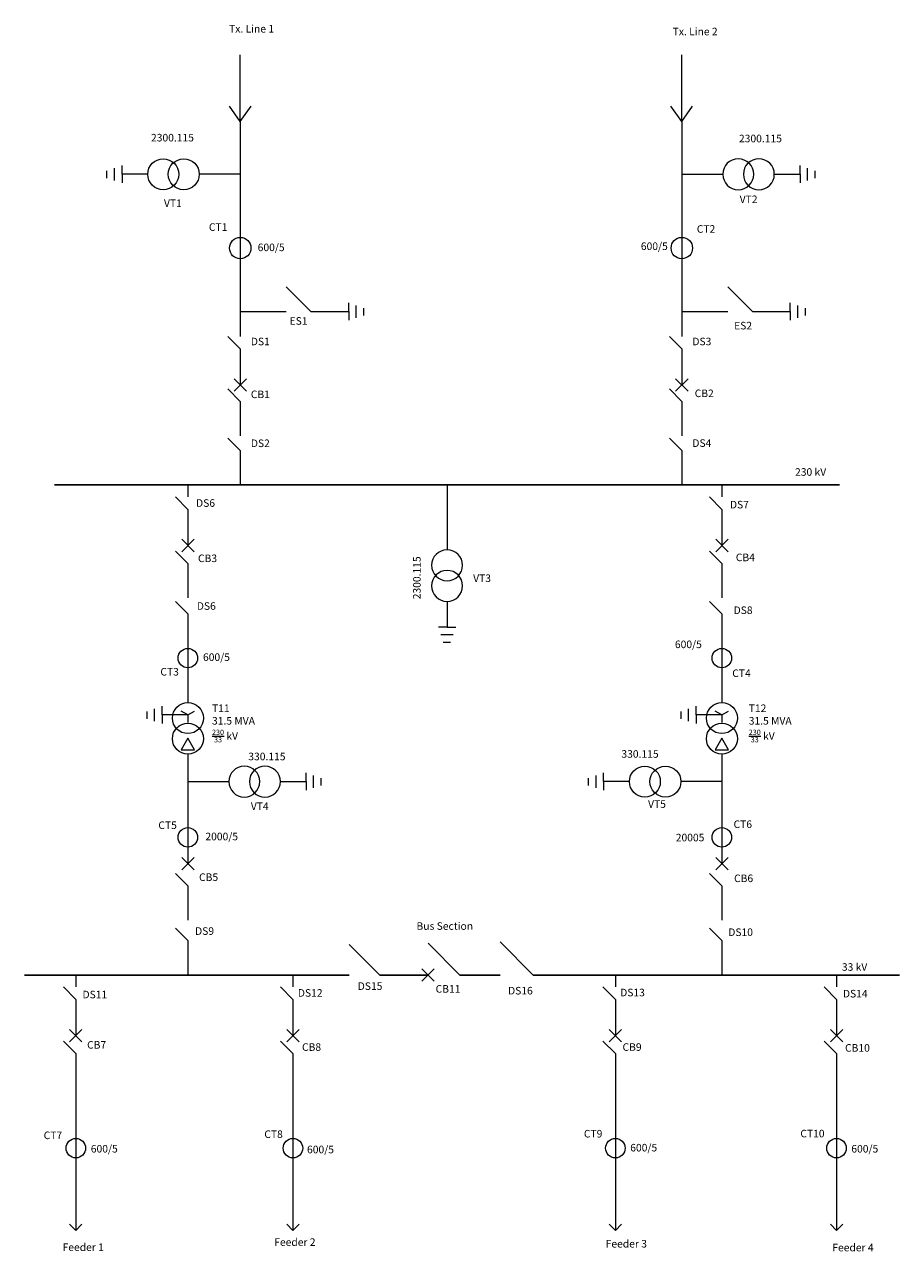
# Model space of a CAD drawing. Units: millimetres. Extents: x 158.9 to 216.7, y 82.5 to 163.7.
import ezdxf

# ---------------------------------------------------------------- set-up
doc = ezdxf.new("R2010")
doc.units = ezdxf.units.MM
doc.header["$MEASUREMENT"] = 0
for name, color, linetype, lineweight in [('E-ANNO-TEXT', 7, 'Continuous', 13), ('E-POWR-BUSB', 7, 'Continuous', 30), ('E-POWR-CKT-HV', 7, 'Continuous', 18), ('E-POWR-CKT-MV', 7, 'Continuous', 18), ('E-POWR-FLOW', 7, 'Continuous', 18), ('E-POWR-INST', 4, 'Continuous', 18), ('E-POWR-SWGR', 3, 'Continuous', 18), ('E-POWR-XFMR', 7, 'Continuous', 20)]:
    doc.layers.add(name, color=color, linetype=linetype, lineweight=lineweight)
doc.styles.get("Standard").update_dxf_attribs({"font": 'arial.ttf'})

# ---------------------------------------------------------------- blocks, each defined once
blk = doc.blocks.new('VT-GROUNDED')
for p, q in [((-8.816, -0.266), (-8.816, 0.233)), ((-8.316, -0.419), (-8.316, 0.402)), ((-7.816, 0), (-7.816, 0.572)), ((-6.117, 0), (-7.816, 0)), ((-7.816, 0), (-7.816, -0.572)), ((0, 0), (-2.709, 0))]:
    blk.add_line(p, q)
for centre in [(-5.093, 0), (-3.733, 0)]:
    blk.add_circle(centre, 1.024)
blk = doc.blocks.new('XFMR-31_5MVA-YN-D')
for p, q in [((-2.699, -0.054), (-2.699, 0.445)), ((-2.199, -0.207), (-2.199, 0.615)), ((-1.699, 0.212), (-1.699, 0.784)), ((0, 0.212), (-1.699, 0.212)), ((-1.699, 0.212), (-1.699, -0.36)), ((0, 0.212), (-0.441, 0.467)), ((0, 0.212), (0.441, 0.467)), ((0, 0.212), (0, -0.297))]:
    blk.add_line(p, q)
blk.add_lwpolyline([(0.441, -2.096), (0, -1.332), (-0.441, -2.096)], close=True)
for centre in [(0, 0), (0, -1.36)]:
    blk.add_circle(centre, 1.024)
blk = doc.blocks.new('SW-EARTH-OPEN')
for p, q in [((4.671, 0), (3.043, 1.628)), ((0, 0), (3.043, 0)), ((4.671, 0), (7.175, 0)), ((7.175, 0), (7.175, 0.572)), ((7.175, 0), (7.175, -0.572)), ((7.675, -0.419), (7.675, 0.402)), ((8.175, -0.266), (8.175, 0.233))]:
    blk.add_line(p, q)
blk = doc.blocks.new('CT-INCOMING')
blk.add_circle((0, 0), 0.707)
blk = doc.blocks.new('CT-BAY')
blk.add_circle((0, 0), 0.644)
blk = doc.blocks.new('DISCONNECT-OPEN')
blk.add_line((0, 0), (-0.823, 0.823))
blk = doc.blocks.new('CB-OPEN-INCOMING')
for p, q in [((-0.409, -0.409), (0.409, 0.409)), ((0.409, -0.409), (-0.409, 0.409)), ((0, -1.078), (-0.823, -0.255))]:
    blk.add_line(p, q)
blk = doc.blocks.new('CB-OPEN-BAY')
for p, q in [((-0.409, -0.409), (0.409, 0.409)), ((0.409, -0.409), (-0.409, 0.409)), ((0, -1.189), (-0.823, -0.365))]:
    blk.add_line(p, q)
blk = doc.blocks.new('CB-OPEN-XFMR-SEC')
for p, q in [((-0.409, -0.409), (0.409, 0.409)), ((0.409, -0.409), (-0.409, 0.409)), ((0, -1.457), (-0.823, -0.634))]:
    blk.add_line(p, q)
blk = doc.blocks.new('FLOW-INCOMING')
for q in [(-0.717, 1.019), (0.717, 1.019)]:
    blk.add_line((0, 0), q)
blk = doc.blocks.new('FLOW-FEEDER')
for q in [(-0.409, 0.409), (0.409, 0.409)]:
    blk.add_line((0, 0), q)

msp = doc.modelspace()

# ---------------------------------------------------------------- linework, layer by layer
at = {"layer": 'E-POWR-BUSB'}
for p, q in [((160.87, 133.206), (212.786, 133.206)), ((158.887, 100.802), (180.357, 100.802)), ((182.371, 100.802), (185.567, 100.802)), ((187.669, 100.802), (190.339, 100.802)), ((192.528, 100.802), (216.742, 100.802))]:
    msp.add_line(p, q, dxfattribs=at)
at = {"layer": 'E-POWR-CKT-HV'}
for p, q in [((173.148, 157.245), (173.148, 161.649)), ((202.35, 157.245), (202.35, 161.649)), ((173.148, 157.245), (173.148, 153.751)), ((202.35, 157.245), (202.35, 153.751)), ((173.148, 153.751), (173.148, 149.575)), ((202.35, 153.751), (202.35, 149.575)), ((173.148, 149.575), (173.148, 143.815)), ((202.35, 149.575), (202.35, 143.815)), ((173.148, 143.815), (173.148, 143.025)), ((202.35, 143.815), (202.35, 143.025)), ((173.148, 142.202), (173.148, 139.812)), ((202.35, 142.202), (202.35, 139.812)), ((173.148, 138.735), (173.148, 136.454)), ((202.35, 138.735), (202.35, 136.454)), ((173.148, 135.487), (173.148, 133.206)), ((202.35, 135.487), (202.35, 133.206)), ((169.687, 133.206), (169.687, 132.416)), ((186.828, 133.206), (186.828, 131.628)), ((204.998, 133.206), (204.998, 132.416)), ((169.687, 131.593), (169.687, 129.204)), ((204.998, 131.593), (204.998, 129.204)), ((169.687, 128.015), (169.687, 125.734)), ((204.998, 128.015), (204.998, 125.734)), ((169.687, 124.683), (169.687, 122.402)), ((204.998, 124.683), (204.998, 122.402)), ((169.687, 122.402), (169.687, 118.814)), ((204.998, 122.402), (204.998, 118.814))]:
    msp.add_line(p, q, dxfattribs=at)
at = {"layer": 'E-POWR-CKT-MV'}
for p, q in [((169.687, 115.406), (169.687, 110.548)), ((204.998, 115.406), (204.998, 110.548)), ((169.687, 110.548), (169.687, 108.158)), ((204.998, 110.548), (204.998, 108.158)), ((169.687, 106.701), (169.687, 104.42)), ((204.998, 106.701), (204.998, 104.42)), ((169.687, 103.083), (169.687, 100.802)), ((204.998, 103.083), (204.998, 100.802)), ((162.276, 100.802), (162.276, 100.011)), ((176.635, 100.802), (176.635, 100.011)), ((197.958, 100.802), (197.958, 100.011)), ((212.581, 100.802), (212.581, 100.011)), ((162.276, 99.188), (162.276, 96.799)), ((176.635, 99.188), (176.635, 96.799)), ((197.958, 99.188), (197.958, 96.799)), ((212.581, 99.188), (212.581, 96.799)), ((162.276, 95.61), (162.276, 90.616)), ((176.635, 95.61), (176.635, 90.693)), ((197.958, 95.61), (197.958, 90.724)), ((212.581, 95.61), (212.581, 90.734)), ((162.276, 92.278), (162.276, 89.997)), ((176.635, 92.278), (176.635, 89.997)), ((197.958, 92.278), (197.958, 89.997)), ((212.581, 92.278), (212.581, 89.997)), ((162.276, 89.997), (162.276, 86.41)), ((176.635, 89.997), (176.635, 86.41)), ((197.958, 89.997), (197.958, 86.41)), ((212.581, 89.997), (212.581, 86.41)), ((162.276, 86.41), (162.276, 83.918)), ((176.635, 86.41), (176.635, 83.918)), ((197.958, 86.41), (197.958, 83.918)), ((212.581, 86.41), (212.581, 83.918))]:
    msp.add_line(p, q, dxfattribs=at)
at = {"layer": 'E-POWR-SWGR'}
for p, q in [((204.589, 128.794), (205.407, 129.613)), ((205.407, 128.794), (204.589, 129.613)), ((182.371, 100.802), (180.357, 102.816)), ((187.669, 100.802), (185.567, 102.903)), ((192.528, 100.802), (190.339, 102.991)), ((185.158, 100.392), (185.976, 101.211)), ((185.976, 100.392), (185.158, 101.211))]:
    msp.add_line(p, q, dxfattribs=at)

# ---------------------------------------------------------------- block references
at = {"layer": 'E-POWR-FLOW'}
for name, p in [('FLOW-INCOMING', (173.148, 157.245)), ('FLOW-INCOMING', (202.35, 157.245)), ('FLOW-FEEDER', (162.276, 83.918)), ('FLOW-FEEDER', (176.635, 83.918)), ('FLOW-FEEDER', (197.958, 83.918)), ('FLOW-FEEDER', (212.581, 83.918))]:
    msp.add_blockref(name, p, dxfattribs=at)
at = {"layer": 'E-POWR-INST'}
for name, p in [('VT-GROUNDED', (173.148, 153.751)), ('CT-INCOMING', (173.148, 148.867)), ('CT-INCOMING', (202.35, 148.867)), ('CT-BAY', (169.687, 121.758)), ('CT-BAY', (204.998, 121.758)), ('VT-GROUNDED', (204.998, 113.59)), ('CT-BAY', (169.687, 109.904)), ('CT-BAY', (204.998, 109.904)), ('CT-BAY', (162.276, 89.354)), ('CT-BAY', (176.635, 89.354)), ('CT-BAY', (197.958, 89.354)), ('CT-BAY', (212.581, 89.354))]:
    msp.add_blockref(name, p, dxfattribs=at)
at = {"layer": 'E-POWR-INST', "extrusion": (0, 0, -1), "zscale": -1}
for p in [(-202.35, 153.751), (-169.687, 113.59)]:
    msp.add_blockref('VT-GROUNDED', p, dxfattribs=at)
at = {"layer": 'E-POWR-INST', "extrusion": (0, 0, -1), "zscale": -1, "rotation": 89.99999999999947}
msp.add_blockref('VT-GROUNDED', (-186.828, 131.628), dxfattribs=at)
at = {"layer": 'E-POWR-SWGR'}
for name, p in [('SW-EARTH-OPEN', (173.148, 144.674)), ('SW-EARTH-OPEN', (202.35, 144.674)), ('DISCONNECT-OPEN', (173.148, 142.202)), ('DISCONNECT-OPEN', (202.35, 142.202)), ('CB-OPEN-INCOMING', (173.148, 139.812)), ('CB-OPEN-INCOMING', (202.35, 139.812)), ('DISCONNECT-OPEN', (173.148, 135.487)), ('DISCONNECT-OPEN', (202.35, 135.487)), ('DISCONNECT-OPEN', (169.687, 131.593)), ('DISCONNECT-OPEN', (204.998, 131.593)), ('CB-OPEN-BAY', (169.687, 129.204)), ('CB-OPEN-BAY', (204.998, 129.204)), ('DISCONNECT-OPEN', (169.687, 124.683)), ('DISCONNECT-OPEN', (204.998, 124.683)), ('CB-OPEN-XFMR-SEC', (169.687, 108.158)), ('CB-OPEN-XFMR-SEC', (204.998, 108.158)), ('DISCONNECT-OPEN', (169.687, 103.083)), ('DISCONNECT-OPEN', (204.998, 103.083)), ('DISCONNECT-OPEN', (162.276, 99.188)), ('DISCONNECT-OPEN', (176.635, 99.188)), ('DISCONNECT-OPEN', (197.958, 99.188)), ('DISCONNECT-OPEN', (212.581, 99.188)), ('CB-OPEN-BAY', (162.276, 96.799)), ('CB-OPEN-BAY', (176.635, 96.799)), ('CB-OPEN-BAY', (197.958, 96.799)), ('CB-OPEN-BAY', (212.581, 96.799))]:
    msp.add_blockref(name, p, dxfattribs=at)
at = {"layer": 'E-POWR-XFMR'}
for p in [(169.687, 117.79), (204.998, 117.79)]:
    msp.add_blockref('XFMR-31_5MVA-YN-D', p, dxfattribs=at)

# ---------------------------------------------------------------- texts
at = {"layer": 'E-ANNO-TEXT', "char_height": 0.5, "attachment_point": 1}
for s, width, insert in [('Tx. Line 1', 3.21529, (172.411, 163.623)), ('Tx. Line 2', 3.21529, (201.743, 163.441)), ('2300.115', 3.21529, (167.249, 156.421)), ('2300.115', 3.21529, (206.129, 156.365)), ('VT1', 3.21529, (168.106, 152.083)), ('VT2', 3.21529, (206.175, 152.347)), ('CT1', 3.21529, (171.076, 150.508)), ('CT2', 3.21529, (203.342, 150.384)), ('600/5', 3.21529, (199.641, 149.243)), ('600/5', 3.21529, (174.304, 149.167)), ('ES1', 3.21529, (176.412, 144.302)), ('ES2', 3.21529, (205.809, 143.993)), ('DS1', 3.21529, (173.851, 142.943)), ('DS3', 3.21529, (203.048, 142.943)), ('CB1', 3.21529, (173.851, 139.448)), ('CB2', 3.21529, (203.202, 139.515)), ('DS2', 3.21529, (173.851, 136.213)), ('DS4', 3.21529, (203.047, 136.225)), ('230 kV', 3.21529, (209.838, 134.315)), ('DS6', 3.21529, (170.228, 132.262)), ('DS7', 3.21529, (205.532, 132.156)), ('CB3', 3.21529, (170.357, 128.606)), ('CB4', 3.21529, (205.92, 128.665)), ('VT3', 3.21529, (188.552, 127.29)), ('DS6', 3.21529, (170.28, 125.451)), ('DS8', 3.21529, (205.774, 125.173)), ('600/5', 3.21529, (201.893, 122.918)), ('600/5', 3.21529, (170.687, 122.07)), ('CT3', 3.21529, (167.869, 121.103)), ('CT4', 3.21529, (205.685, 121.008)), ('\\A1;T11\\P31.5 MVA\\P{\\H0.7x;\\S230/33;} kV', 3.21529, (171.284, 118.693)), ('\\A1;T12\\P31.5 MVA\\P{\\H0.7x;\\S230/33;} kV', 3.21529, (206.775, 118.693)), ('330.115', 3.21529, (173.683, 115.502)), ('330.115', 3.21529, (198.355, 115.669)), ('VT4', 3.21529, (173.851, 112.213)), ('VT5', 3.21529, (200.118, 112.353)), ('CT5', 3.21529, (167.736, 110.958)), ('CT6', 3.21529, (205.771, 111.022)), ('2000/5', 3.21529, (170.846, 110.211)), ('20005', 3.21529, (201.95, 110.142)), ('CB5', 3.21529, (170.427, 107.521)), ('CB6', 3.21529, (205.805, 107.446)), ('DS9', 3.21529, (170.165, 103.959)), ('Bus Section', 4.47822, (184.805, 104.29)), ('DS10', 3.21529, (205.42, 103.883)), ('33 kV', 3.21529, (212.935, 101.582)), ('DS12', 3.21529, (176.959, 99.867)), ('DS15', 3.21529, (180.919, 100.317)), ('CB11', 3.21529, (186.07, 100.136)), ('DS16', 3.21529, (190.86, 100.016)), ('DS13', 3.21529, (198.274, 99.894)), ('DS14', 3.21529, (213.004, 99.819)), ('DS11', 3.21529, (162.719, 99.761)), ('CB7', 3.21529, (163.024, 96.434)), ('CB8', 3.21529, (177.235, 96.288)), ('CB9', 3.21529, (198.429, 96.289)), ('CB10', 3.21529, (213.144, 96.234)), ('CT7', 3.21529, (160.152, 90.45)), ('CT8', 3.21529, (174.742, 90.526)), ('CT9', 3.21529, (195.874, 90.558)), ('CT10', 3.21529, (210.189, 90.568)), ('600/5', 3.21529, (163.269, 89.564)), ('600/5', 3.21529, (177.566, 89.514)), ('600/5', 3.21529, (198.939, 89.635)), ('600/5', 3.21529, (213.558, 89.563)), ('Feeder 1', 3.21529, (161.404, 83.053)), ('Feeder 2', 3.21529, (175.398, 83.389)), ('Feeder 3', 3.21529, (197.315, 83.282)), ('Feeder 4', 3.21529, (212.301, 83.031))]:
    msp.add_mtext_dynamic_manual_height_columns(s, width=width, gutter_width=1, heights=[0], dxfattribs=dict(at, insert=insert))
at = {"layer": 'E-ANNO-TEXT', "insert": (184.579, 125.648), "char_height": 0.5, "attachment_point": 1, "rotation": 90}
msp.add_mtext_dynamic_manual_height_columns('2300.115', width=3.21529, gutter_width=1, heights=[0], dxfattribs=at)

doc.saveas('drawing.dxf')
